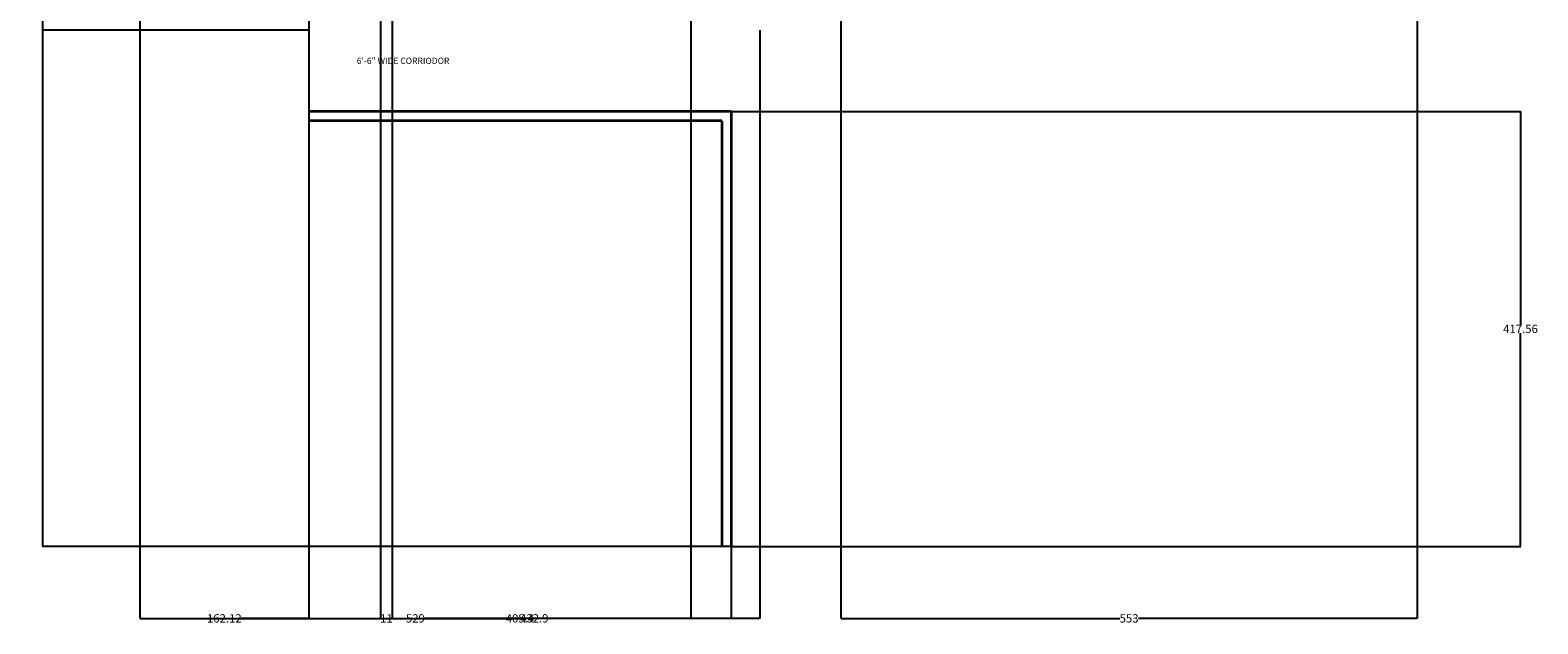
# Model space of a CAD drawing. Units: inches. Extents: x 3343 to 4790, y 1140 to 2641.
# Tile 1 of 10: x 3343 to 4790, y 1140 to 1710. Entities that reach past the tile are written whole.
import ezdxf

# ---------------------------------------------------------------- set-up
doc = ezdxf.new("R2010")
doc.units = ezdxf.units.IN
doc.header["$LTSCALE"] = 5
doc.header["$MEASUREMENT"] = 0
for name, color, linetype, lineweight in [('A-ANNO-DIMS', 2, 'Continuous', 18), ('A-AREA-IDEN', 7, 'Continuous', 18), ('A-WALL', 7, 'Continuous', 35)]:
    doc.layers.add(name, color=color, linetype=linetype, lineweight=lineweight)
doc.styles.get("Standard").update_dxf_attribs({"font": 'arial.ttf'})
doc.dimstyles.get("Standard").update_dxf_attribs({"dimtxt": 8, "dimasz": 0.18, "dimexe": 0.18, "dimexo": 0.0625, "dimgap": 0.09, "dimtad": 0, "dimtih": 1, "dimtoh": 1, "dimdec": 1, "dimzin": 0, "dimdsep": 46, "dimlunit": 3, "dimtxsty": 'Standard', "dimcen": 0.09, "dimadec": 0, "dimazin": 0, "dimtfac": 1, "dimtdec": 1, "dimtofl": 0, "dimtmove": 0, "dimatfit": 3, "dimfxl": 1, "dimtolj": 1, "dimtzin": 0, "dimarcsym": 0})

# ---------------------------------------------------------------- blocks, each defined once
blk = doc.blocks.new('*D84')
at = {"layer": 'A-ANNO-DIMS', "color": 0, "lineweight": -2, "ltscale": 5, "transparency": 16777216}
for p, q in [((3448.1, 2566.2), (3354.8, 2566.2)), ((3355, 2566), (3355, 1894.3)), ((3355, 1214.3), (3355, 1886)), ((4015.6, 1214.1), (3354.8, 1214.1))]:
    blk.add_line(p, q, dxfattribs=at)
at = {"layer": 'A-ANNO-DIMS', "color": 0, "ltscale": 5, "transparency": 16777216}
for points in [[(3354.9, 2566), (3355, 2566), (3355, 2566.2)], [(3354.9, 1214.3), (3355, 1214.3), (3355, 1214.1)]]:
    blk.add_solid(points, dxfattribs=at)
at = {"layer": 'Defpoints', "color": 0, "ltscale": 5, "transparency": 16777216}
for p in [(3448.1, 2566.2), (3355, 1214.1), (4015.6, 1214.1)]:
    blk.add_point(p, dxfattribs=at)
at = {"layer": 'A-ANNO-DIMS', "color": 0, "ltscale": 5, "transparency": 16777216, "insert": (3355, 1890.1), "char_height": 8, "attachment_point": 5}
blk.add_mtext('\\A1;1352', dxfattribs=at)
blk = doc.blocks.new('*D85')
at = {"layer": 'A-ANNO-DIMS', "color": 0, "lineweight": -2, "ltscale": 5, "transparency": 16777216}
for p, q in [((3448.1, 2014.1), (3448.1, 1144.8)), ((3977.1, 2014.1), (3977.1, 1144.8)), ((3448.3, 1145), (3703.7, 1145)), ((3976.9, 1145), (3721.6, 1145))]:
    blk.add_line(p, q, dxfattribs=at)
at = {"layer": 'A-ANNO-DIMS', "color": 0, "ltscale": 5, "transparency": 16777216}
for points in [[(3448.3, 1145), (3448.3, 1144.9), (3448.1, 1145)], [(3976.9, 1145), (3976.9, 1144.9), (3977.1, 1145)]]:
    blk.add_solid(points, dxfattribs=at)
at = {"layer": 'Defpoints', "color": 0, "ltscale": 5, "transparency": 16777216}
for p in [(3448.1, 2014.2), (3977.1, 2014.2), (3977.1, 1145)]:
    blk.add_point(p, dxfattribs=at)
at = {"layer": 'A-ANNO-DIMS', "color": 0, "ltscale": 5, "transparency": 16777216, "insert": (3712.6, 1145), "char_height": 8, "attachment_point": 5}
blk.add_mtext('\\A1;529', dxfattribs=at)
blk = doc.blocks.new('*D86')
at = {"layer": 'A-ANNO-DIMS', "color": 0, "lineweight": -2, "ltscale": 5, "transparency": 16777216}
for p, q in [((4121.1, 1851.1), (4121.1, 1144.8)), ((4674.1, 1851.1), (4674.1, 1144.8)), ((4121.3, 1145), (4388.7, 1145)), ((4673.9, 1145), (4406.6, 1145))]:
    blk.add_line(p, q, dxfattribs=at)
at = {"layer": 'A-ANNO-DIMS', "color": 0, "ltscale": 5, "transparency": 16777216}
for points in [[(4121.3, 1145), (4121.3, 1144.9), (4121.1, 1145)], [(4673.9, 1145), (4673.9, 1144.9), (4674.1, 1145)]]:
    blk.add_solid(points, dxfattribs=at)
at = {"layer": 'Defpoints', "color": 0, "ltscale": 5, "transparency": 16777216}
for p in [(4121.1, 1851.2), (4674.1, 1851.2), (4674.1, 1145)]:
    blk.add_point(p, dxfattribs=at)
at = {"layer": 'A-ANNO-DIMS', "color": 0, "ltscale": 5, "transparency": 16777216, "insert": (4397.6, 1145), "char_height": 8, "attachment_point": 5}
blk.add_mtext('\\A1;553', dxfattribs=at)
blk = doc.blocks.new('*D90')
at = {"layer": 'A-ANNO-DIMS', "color": 0, "lineweight": -2, "ltscale": 5, "transparency": 16777216}
for p, q in [((3610.2, 1841.7), (3354.8, 1841.7)), ((3355, 1841.5), (3355, 1779.8)), ((3355, 1709.8), (3355, 1771.5)), ((3610.2, 1709.7), (3354.8, 1709.7))]:
    blk.add_line(p, q, dxfattribs=at)
at = {"layer": 'A-ANNO-DIMS', "color": 0, "ltscale": 5, "transparency": 16777216}
for points in [[(3354.9, 1841.5), (3355, 1841.5), (3355, 1841.7)], [(3354.9, 1709.8), (3355, 1709.8), (3355, 1709.7)]]:
    blk.add_solid(points, dxfattribs=at)
at = {"layer": 'Defpoints', "color": 0, "ltscale": 5, "transparency": 16777216}
for p in [(3355, 1841.7), (3610.2, 1841.7), (3610.2, 1709.7)]:
    blk.add_point(p, dxfattribs=at)
at = {"layer": 'A-ANNO-DIMS', "color": 0, "ltscale": 5, "transparency": 16777216, "insert": (3355, 1775.7), "char_height": 8, "attachment_point": 5}
blk.add_mtext('\\A1;132', dxfattribs=at)
blk = doc.blocks.new('*D91')
at = {"layer": 'A-ANNO-DIMS', "color": 0, "lineweight": -2, "ltscale": 5, "transparency": 16777216}
for p, q in [((3610.2, 1709.6), (3610.2, 1144.8)), ((4043.1, 1709.6), (4043.1, 1144.8)), ((3610.4, 1145), (3812.9, 1145)), ((4042.9, 1145), (3840.4, 1145))]:
    blk.add_line(p, q, dxfattribs=at)
at = {"layer": 'A-ANNO-DIMS', "color": 0, "ltscale": 5, "transparency": 16777216}
for points in [[(3610.4, 1145), (3610.4, 1144.9), (3610.2, 1145)], [(4042.9, 1145), (4042.9, 1144.9), (4043.1, 1145)]]:
    blk.add_solid(points, dxfattribs=at)
at = {"layer": 'Defpoints', "color": 0, "ltscale": 5, "transparency": 16777216}
for p in [(3610.2, 1709.7), (4043.1, 1709.7), (4043.1, 1145)]:
    blk.add_point(p, dxfattribs=at)
at = {"layer": 'A-ANNO-DIMS', "color": 0, "ltscale": 5, "transparency": 16777216, "insert": (3826.7, 1145), "char_height": 8, "attachment_point": 5}
blk.add_mtext('\\A1;432.9', dxfattribs=at)
blk = doc.blocks.new('*D92')
at = {"layer": 'A-ANNO-DIMS', "color": 0, "lineweight": -2, "ltscale": 5, "transparency": 16777216}
for p, q in [((3610.2, 1622.6), (3610.2, 1144.8)), ((4015.6, 1631.6), (4015.6, 1144.8)), ((3610.4, 1145), (3799.2, 1145)), ((4015.5, 1145), (3826.7, 1145))]:
    blk.add_line(p, q, dxfattribs=at)
at = {"layer": 'A-ANNO-DIMS', "color": 0, "ltscale": 5, "transparency": 16777216}
for points in [[(3610.4, 1145), (3610.4, 1144.9), (3610.2, 1145)], [(4015.5, 1145), (4015.5, 1144.9), (4015.6, 1145)]]:
    blk.add_solid(points, dxfattribs=at)
at = {"layer": 'Defpoints', "color": 0, "ltscale": 5, "transparency": 16777216}
for p in [(3610.2, 1622.7), (4015.6, 1631.7), (4015.6, 1145)]:
    blk.add_point(p, dxfattribs=at)
at = {"layer": 'A-ANNO-DIMS', "color": 0, "ltscale": 5, "transparency": 16777216, "insert": (3812.9, 1145), "char_height": 8, "attachment_point": 5}
blk.add_mtext('\\A1;405.4', dxfattribs=at)
blk = doc.blocks.new('*D93')
at = {"layer": 'A-ANNO-DIMS', "color": 0, "lineweight": -2, "ltscale": 5, "transparency": 16777216}
for p, q in [((4015.7, 1631.7), (4773.5, 1631.7)), ((4773.3, 1631.5), (4773.3, 1427.1)), ((4773.3, 1214.3), (4773.3, 1418.7)), ((4015.7, 1214.1), (4773.5, 1214.1))]:
    blk.add_line(p, q, dxfattribs=at)
at = {"layer": 'A-ANNO-DIMS', "color": 0, "ltscale": 5, "transparency": 16777216}
for points in [[(4773.2, 1631.5), (4773.3, 1631.5), (4773.3, 1631.7)], [(4773.2, 1214.3), (4773.3, 1214.3), (4773.3, 1214.1)]]:
    blk.add_solid(points, dxfattribs=at)
at = {"layer": 'Defpoints', "color": 0, "ltscale": 5, "transparency": 16777216}
for p in [(4015.6, 1631.7), (4773.3, 1631.7), (4015.6, 1214.1)]:
    blk.add_point(p, dxfattribs=at)
at = {"layer": 'A-ANNO-DIMS', "color": 0, "ltscale": 5, "transparency": 16777216, "insert": (4773.3, 1422.9), "char_height": 8, "attachment_point": 5}
blk.add_mtext('\\A1;417.56', dxfattribs=at)
blk = doc.blocks.new('*D94')
at = {"layer": 'A-ANNO-DIMS', "color": 0, "lineweight": -2, "ltscale": 5, "transparency": 16777216}
for p, q in [((3448.1, 2014.1), (3448.1, 1144.8)), ((3610.2, 1841.6), (3610.2, 1144.8)), ((3448.3, 1145), (3512.9, 1145)), ((3610.1, 1145), (3545.5, 1145))]:
    blk.add_line(p, q, dxfattribs=at)
at = {"layer": 'A-ANNO-DIMS', "color": 0, "ltscale": 5, "transparency": 16777216}
for points in [[(3448.3, 1145), (3448.3, 1144.9), (3448.1, 1145)], [(3610.1, 1145), (3610.1, 1144.9), (3610.2, 1145)]]:
    blk.add_solid(points, dxfattribs=at)
at = {"layer": 'Defpoints', "color": 0, "ltscale": 5, "transparency": 16777216}
for p in [(3448.1, 2014.2), (3610.2, 1841.7), (3610.2, 1145)]:
    blk.add_point(p, dxfattribs=at)
at = {"layer": 'A-ANNO-DIMS', "color": 0, "ltscale": 5, "transparency": 16777216, "insert": (3529.2, 1145), "char_height": 8, "attachment_point": 5}
blk.add_mtext('\\A1;162.12', dxfattribs=at)
blk = doc.blocks.new('*D97')
at = {"layer": 'A-ANNO-DIMS', "color": 0, "lineweight": -2, "ltscale": 5, "transparency": 16777216}
for p, q in [((3679.2, 1718.6), (3679.2, 1144.8)), ((3690.2, 1718.6), (3690.2, 1144.8)), ((3679.4, 1145), (3680.1, 1145)), ((3690.1, 1145), (3689.4, 1145))]:
    blk.add_line(p, q, dxfattribs=at)
at = {"layer": 'A-ANNO-DIMS', "color": 0, "ltscale": 5, "transparency": 16777216}
for points in [[(3679.4, 1145), (3679.4, 1144.9), (3679.2, 1145)], [(3690.1, 1145), (3690.1, 1144.9), (3690.2, 1145)]]:
    blk.add_solid(points, dxfattribs=at)
at = {"layer": 'Defpoints', "color": 0, "ltscale": 5, "transparency": 16777216}
for p in [(3679.2, 1718.7), (3690.2, 1718.7), (3690.2, 1145)]:
    blk.add_point(p, dxfattribs=at)
at = {"layer": 'A-ANNO-DIMS', "color": 0, "ltscale": 5, "transparency": 16777216, "insert": (3684.7, 1145), "char_height": 8, "attachment_point": 5}
blk.add_mtext('\\A1;11', dxfattribs=at)

msp = doc.modelspace()

# ---------------------------------------------------------------- linework, layer by layer
at = {"layer": 'A-WALL', "ltscale": 5}
for p, q in [((4015.647, 1631.669), (3610.248, 1631.669)), ((4006.647, 1622.669), (3610.248, 1622.669)), ((4006.647, 1622.669), (4006.647, 1214.112)), ((4015.647, 1631.669), (4015.647, 1214.112))]:
    msp.add_line(p, q, dxfattribs=at)

# ---------------------------------------------------------------- texts
at = {"layer": 'A-AREA-IDEN', "ltscale": 5, "insert": (3656.375, 1683.227), "char_height": 6, "attachment_point": 1}
msp.add_mtext_dynamic_manual_height_columns('6\'-6" WIDE CORRIODOR', width=189.69543, gutter_width=1, heights=[0], dxfattribs=at)

# ---------------------------------------------------------------- dimensions: what is measured, and where the dimension line sits
at = {"layer": 'A-ANNO-DIMS', "ltscale": 5}
for base, p1, p2, override, picture, middle in [((3354.98, 1214.112), (3448.13, 2566.161), (4015.647, 1214.112), {"dimdec": 0, "dimlfac": 1, "dimrnd": 0, "dimzin": 0, "dimdsep": 46, "dimlunit": 2}, '*D84', (3354.98, 1890.137)), ((3354.98, 1841.669), (3610.248, 1709.669), (3610.248, 1841.669), {"dimdec": 0, "dimlfac": 1, "dimrnd": 0, "dimzin": 0, "dimdsep": 46, "dimlunit": 2}, '*D90', (3354.98, 1775.669)), ((4773.28, 1631.669), (4015.647, 1214.112), (4015.647, 1631.669), {"dimdec": 2, "dimlfac": 1, "dimrnd": 0, "dimzin": 0, "dimdsep": 46, "dimlunit": 2}, '*D93', (4773.28, 1422.891))]:
    dim = msp.add_linear_dim(base=base, p1=p1, p2=p2, angle=90, dimstyle='Standard', override=override, dxfattribs=at)
    dim.commit()
    dim.dimension.update_dxf_attribs({"geometry": picture, "text_midpoint": middle})
for base, p1, p2, override, picture, middle in [((3977.13, 1144.962), (3448.13, 2014.161), (3977.13, 2014.161), {"dimdec": 0, "dimlfac": 1, "dimrnd": 0, "dimzin": 0, "dimdsep": 46, "dimlunit": 2}, '*D85', (3712.63, 1144.962)), ((3610.248, 1144.962), (3448.13, 2014.161), (3610.248, 1841.669), {"dimdec": 2, "dimlfac": 1, "dimrnd": 0, "dimzin": 0, "dimdsep": 46, "dimlunit": 2}, '*D94', (3529.189, 1144.962)), ((4674.13, 1144.962), (4121.13, 1851.161), (4674.13, 1851.161), {"dimdec": 0, "dimlfac": 1, "dimrnd": 0, "dimzin": 0, "dimdsep": 46, "dimlunit": 2}, '*D86', (4397.63, 1144.962)), ((4043.13, 1144.962), (3610.248, 1709.669), (4043.13, 1709.669), {"dimdec": 1, "dimlfac": 1, "dimrnd": 0, "dimzin": 0, "dimdsep": 46, "dimlunit": 2}, '*D91', (3826.689, 1144.962)), ((3690.248, 1144.962), (3679.248, 1718.669), (3690.248, 1718.669), {"dimdec": 0, "dimlfac": 1, "dimrnd": 0, "dimzin": 0, "dimdsep": 46, "dimlunit": 2}, '*D97', (3684.748, 1144.962)), ((4015.647, 1144.962), (3610.248, 1622.669), (4015.647, 1631.669), {"dimdec": 1, "dimlfac": 1, "dimrnd": 0, "dimzin": 0, "dimdsep": 46, "dimlunit": 2}, '*D92', (3812.947, 1144.962))]:
    dim = msp.add_linear_dim(base=base, p1=p1, p2=p2, dimstyle='Standard', override=override, dxfattribs=at)
    dim.commit()
    dim.dimension.update_dxf_attribs({"geometry": picture, "text_midpoint": middle})

doc.saveas('drawing.dxf')
